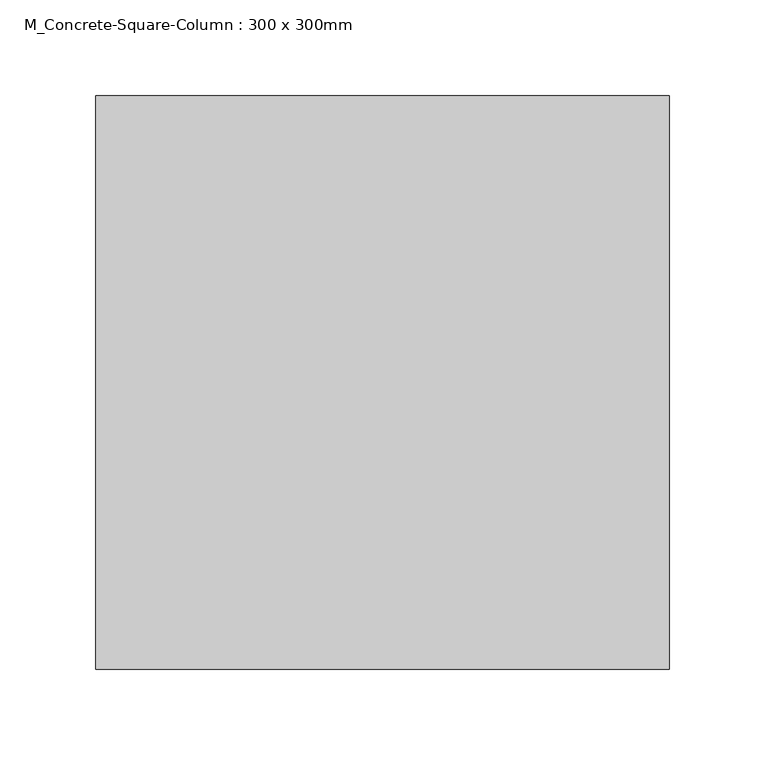
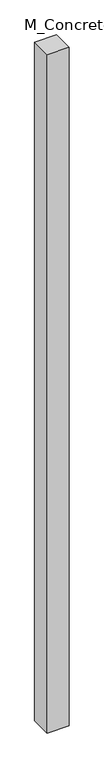
"""IFC4 building model written with IfcOpenShell, lengths in millimetres: column geometry, M_Concrete-Square-Column : 300 x 300mm."""

from ifc_helpers import new_model, si_unit, frame, origin, place, context, project, spatial, polyline, outline, extrude, source, transform, mapped, element, save


def m_concrete_square_column_300_x_300mm_500808f7(model_context):
    return source(origin(), model_context, "Body", "SweptSolid", [
        extrude(outline(polyline([(150.0, 150.0), (150.0, -150.0), (-150.0, -150.0), (-150.0, 150.0), (150.0, 150.0)])), frame((0.0, 0.0, -457.2), z_axis=(0.0, 0.0, 1.0), x_axis=(1.0, 0.0, 0.0)), (0.0, 0.0, 1.0), 9906.0),
    ])


if __name__ == "__main__":
    model = new_model("IFC4")
    model_context = context("Model", 3, world=origin())
    ifc_project = project(units=[si_unit("LENGTHUNIT", "METRE", prefix="MILLI")], contexts=[model_context])
    site = spatial("IfcSite", under=ifc_project)
    building = spatial("IfcBuilding", under=site)
    placement = place(None, origin())
    m_concrete_square_column_300_x_300mm_shape = m_concrete_square_column_300_x_300mm_500808f7(model_context)
    element("IfcColumn", 1, ObjectType="M_Concrete-Square-Column : 300 x 300mm", at=placement, inside=building, context=model_context, shape_type="MappedRepresentation", body=[
        mapped(m_concrete_square_column_300_x_300mm_shape, transform((0.0, 0.0, 0.0), x_axis=(1.0, 0.0, 0.0), y_axis=(0.0, 1.0, 0.0), z_axis=(0.0, 0.0, 1.0))),
    ])
    save(model, "model.ifc")

# Revit data of these elements
# Type "M_Concrete-Square-Column : 300 x 300mm"
#   b = 0.984252 ft
#   Structural Material [instance default] = Concrete, Cast-in-Place gray
# Element 1 (IfcColumn, "M_Concrete-Square-Column : 300 x 300mm")
#   Materials on its faces: "Concrete, Cast-in-Place gray"
# Materials
#   "Concrete, Cast-in-Place gray": class "Concrete", colour RGB 192 192 192, transparency 0, Description = "Cast-in-place concrete", Cost = 0
